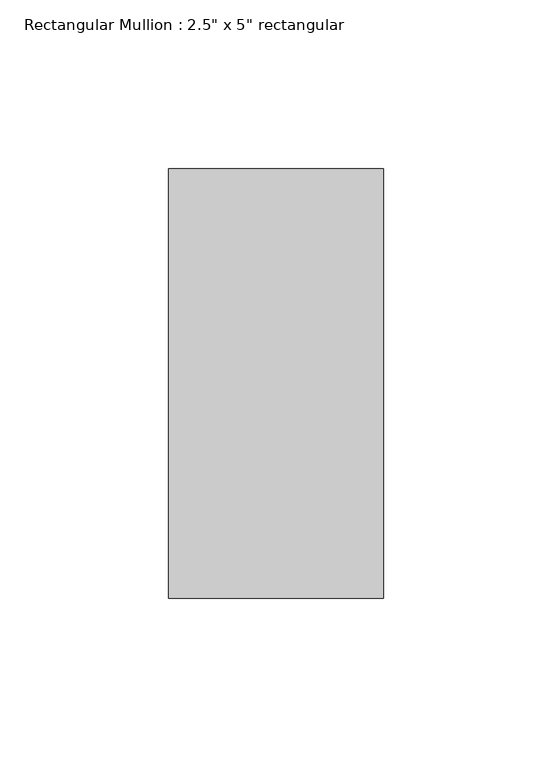
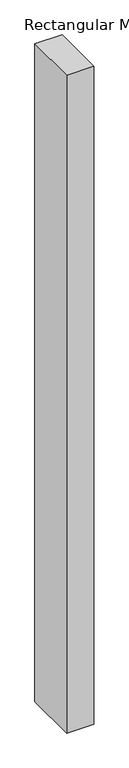
"""IFC4 building model written with IfcOpenShell, lengths in millimetres: member geometry."""

from ifc_helpers import new_model, si_unit, frame, origin, place, context, project, spatial, polyline, outline, extrude, source, transform, mapped, element, save


def member_df09edd1(model_context):
    return source(origin(), model_context, "Body", "SweptSolid", [
        extrude(outline(polyline([(31.75, 63.5), (31.75, -63.5), (-31.75, -63.5), (-31.75, 63.5), (31.75, 63.5)])), frame((0.0, 0.0, -1611.7177577), z_axis=(0.0, 0.0, 1.0), x_axis=(1.0, 0.0, 0.0)), (0.0, 0.0, 1.0), 1611.7177577),
    ])


if __name__ == "__main__":
    model = new_model("IFC4")
    model_context = context("Model", 3, world=origin())
    ifc_project = project(units=[si_unit("LENGTHUNIT", "METRE", prefix="MILLI")], contexts=[model_context])
    site = spatial("IfcSite", under=ifc_project)
    building = spatial("IfcBuilding", under=site)
    placement = place(None, origin())
    member_shape = member_df09edd1(model_context)
    element("IfcMember", 1, ObjectType="Rectangular Mullion : 2.5\" x 5\" rectangular", at=placement, inside=building, context=model_context, shape_type="MappedRepresentation", body=[
        mapped(member_shape, transform((0.0, 0.0, 0.0), x_axis=(1.0, 0.0, 0.0), y_axis=(0.0, 1.0, 0.0), z_axis=(0.0, 0.0, 1.0))),
    ])
    save(model, "model.ifc")

# Revit data of these elements
# Type "Rectangular Mullion : 2.5\" x 5\" rectangular"
#   built-in parameter 1007304 = 0.416667 (stored number, unit not read)
#   built-in parameter 1007301 = 0.104167 (stored number, unit not read)
#   built-in parameter 1007300 = 0.104167 (stored number, unit not read)
# Element 1 (IfcMember, "Rectangular Mullion : 2.5\" x 5\" rectangular")
#   Materials on its faces: "Aluminum"
# Materials
#   "Aluminum": class "Metal", colour RGB 247 247 247, transparency 0, Description = "Aluminum 6061", Cost = 0
